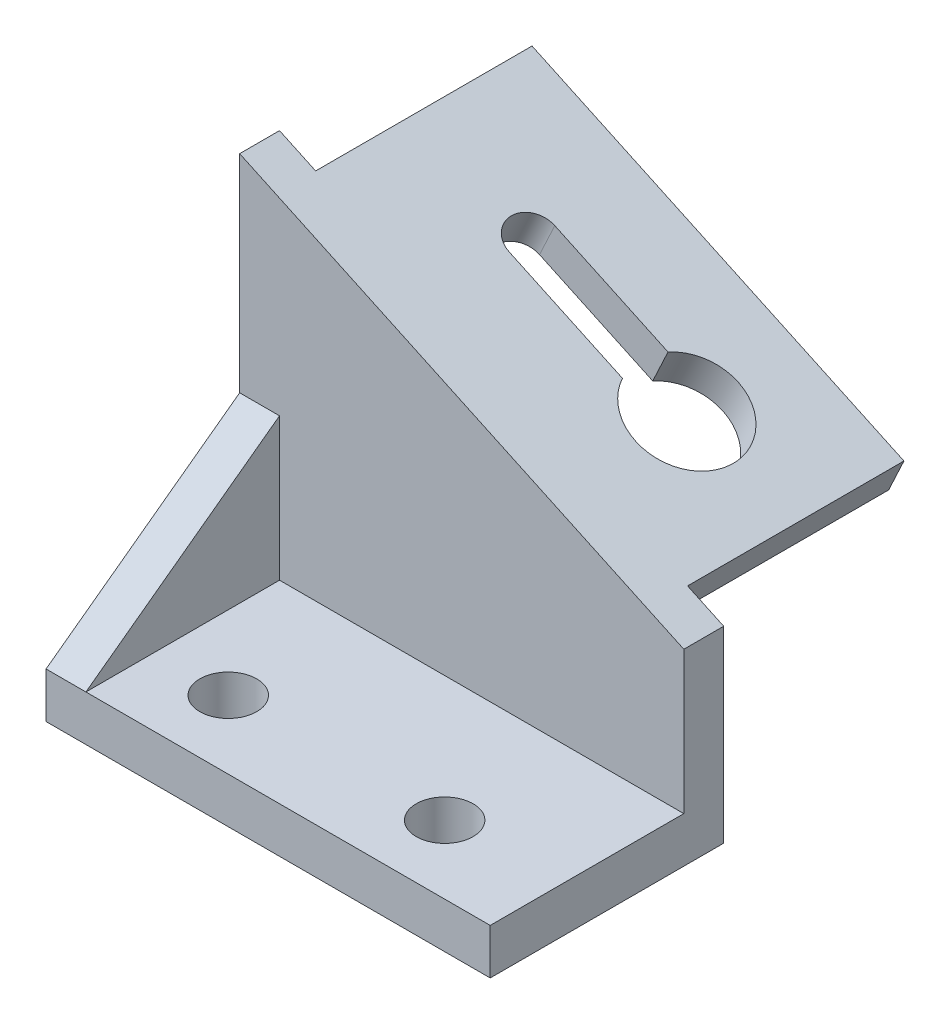
ISO-10303-21;
HEADER;
FILE_DESCRIPTION(('STEP AP214'),'2;1');
FILE_NAME('part.step','',(''),(''),'','','');
FILE_SCHEMA(('AUTOMOTIVE_DESIGN { 1 0 10303 214 1 1 1 1 }'));
ENDSEC;
DATA;
#1=APPLICATION_CONTEXT('core data for automotive mechanical design processes');
#2=APPLICATION_PROTOCOL_DEFINITION('international standard','automotive_design',2000,#1);
#3=PRODUCT_CONTEXT('',#1,'mechanical');
#4=PRODUCT('Part','Part','',(#3));
#5=PRODUCT_RELATED_PRODUCT_CATEGORY('part','',(#4));
#6=PRODUCT_DEFINITION_FORMATION('','',#4);
#7=PRODUCT_DEFINITION_CONTEXT('part definition',#1,'design');
#8=PRODUCT_DEFINITION('design','',#6,#7);
#9=PRODUCT_DEFINITION_SHAPE('','',#8);
#10=(LENGTH_UNIT() NAMED_UNIT(*) SI_UNIT(.MILLI.,.METRE.));
#11=(NAMED_UNIT(*) PLANE_ANGLE_UNIT() SI_UNIT($,.RADIAN.));
#12=(NAMED_UNIT(*) SI_UNIT($,.STERADIAN.) SOLID_ANGLE_UNIT());
#13=UNCERTAINTY_MEASURE_WITH_UNIT(LENGTH_MEASURE(1.E-05),#10,'distance_accuracy_value','');
#14=(GEOMETRIC_REPRESENTATION_CONTEXT(3) GLOBAL_UNCERTAINTY_ASSIGNED_CONTEXT((#13)) GLOBAL_UNIT_ASSIGNED_CONTEXT((#10,
#11,#12)) REPRESENTATION_CONTEXT('',''));
#15=CARTESIAN_POINT('',(0.,0.,0.));
#16=DIRECTION('',(0.,0.,1.));
#17=DIRECTION('',(1.,0.,0.));
#18=AXIS2_PLACEMENT_3D('',#15,#16,#17);
#19=CARTESIAN_POINT('',(-39.,8.,-16.5));
#20=DIRECTION('',(0.,0.,1.));
#21=DIRECTION('',(1.,0.,0.));
#22=AXIS2_PLACEMENT_3D('',#19,#20,#21);
#23=PLANE('',#22);
#24=DIRECTION('',(-0.90630778703665,0.4226182617407,0.));
#25=VECTOR('',#24,1.);
#26=CARTESIAN_POINT('',(39.,26.,-16.5));
#27=LINE('',#26,#25);
#28=CARTESIAN_POINT('',(29.974689939827,30.208571198282,-16.5));
#29=VERTEX_POINT('',#28);
#30=CARTESIAN_POINT('',(-35.3370010416599,60.6639128700022,-16.5));
#31=VERTEX_POINT('',#30);
#32=EDGE_CURVE('E205',#29,#31,#27,.T.);
#33=ORIENTED_EDGE('',*,*,#32,.F.);
#34=DIRECTION('',(0.4226182617407,0.906307787036649,0.));
#35=VECTOR('',#34,1.);
#36=CARTESIAN_POINT('',(16.5963515445968,1.51863192479222,-16.5));
#37=LINE('',#36,#35);
#38=CARTESIAN_POINT('',(32.6558454907434,35.9583278321849,-16.5));
#39=VERTEX_POINT('',#38);
#40=EDGE_CURVE('E195',#29,#39,#37,.T.);
#41=ORIENTED_EDGE('',*,*,#40,.T.);
#42=DIRECTION('',(0.90630778703665,-0.4226182617407,0.));
#43=VECTOR('',#42,1.);
#44=CARTESIAN_POINT('',(41.6811555509164,31.7497566339029,-16.5));
#45=LINE('',#44,#43);
#46=CARTESIAN_POINT('',(39.,33.,-16.5));
#47=VERTEX_POINT('',#46);
#48=EDGE_CURVE('E189',#39,#47,#45,.T.);
#49=ORIENTED_EDGE('',*,*,#48,.T.);
#50=DIRECTION('',(0.,-1.,0.));
#51=VECTOR('',#50,1.);
#52=CARTESIAN_POINT('',(39.,8.,-16.5));
#53=LINE('',#52,#51);
#54=CARTESIAN_POINT('',(39.,0.,-16.5));
#55=VERTEX_POINT('',#54);
#56=EDGE_CURVE('E276',#47,#55,#53,.T.);
#57=ORIENTED_EDGE('',*,*,#56,.T.);
#58=DIRECTION('',(-1.,0.,0.));
#59=VECTOR('',#58,1.);
#60=CARTESIAN_POINT('',(-39.,0.,-16.5));
#61=LINE('',#60,#59);
#62=CARTESIAN_POINT('',(-39.,0.,-16.5));
#63=VERTEX_POINT('',#62);
#64=EDGE_CURVE('E266',#55,#63,#61,.T.);
#65=ORIENTED_EDGE('',*,*,#64,.T.);
#66=DIRECTION('',(0.,-1.,0.));
#67=VECTOR('',#66,1.);
#68=CARTESIAN_POINT('',(-39.,8.,-16.5));
#69=LINE('',#68,#67);
#70=CARTESIAN_POINT('',(-39.,69.37199733609,-16.5));
#71=VERTEX_POINT('',#70);
#72=EDGE_CURVE('E277',#71,#63,#69,.T.);
#73=ORIENTED_EDGE('',*,*,#72,.F.);
#74=DIRECTION('',(0.90630778703665,-0.4226182617407,0.));
#75=VECTOR('',#74,1.);
#76=CARTESIAN_POINT('',(-32.6558454907434,66.4136695039051,-16.5));
#77=LINE('',#76,#75);
#78=CARTESIAN_POINT('',(-32.6558454907434,66.4136695039051,-16.5));
#79=VERTEX_POINT('',#78);
#80=EDGE_CURVE('E186',#71,#79,#77,.T.);
#81=ORIENTED_EDGE('',*,*,#80,.T.);
#82=DIRECTION('',(0.4226182617407,0.906307787036649,0.));
#83=VECTOR('',#82,1.);
#84=CARTESIAN_POINT('',(-48.7153394368901,31.9739735965124,-16.5));
#85=LINE('',#84,#83);
#86=EDGE_CURVE('E162',#31,#79,#85,.T.);
#87=ORIENTED_EDGE('',*,*,#86,.F.);
#88=EDGE_LOOP('',(#33,#41,#49,#57,#65,#73,#81,#87));
#89=FACE_BOUND('',#88,.T.);
#90=ADVANCED_FACE('F39',(#89),#23,.F.);
#91=CARTESIAN_POINT('',(0.,8.,0.));
#92=DIRECTION('',(0.,-1.,0.));
#93=DIRECTION('',(0.,0.,-1.));
#94=AXIS2_PLACEMENT_3D('',#91,#92,#93);
#95=PLANE('',#94);
#96=CARTESIAN_POINT('',(19.,8.,12.5));
#97=DIRECTION('',(0.,1.,0.));
#98=DIRECTION('',(0.,0.,1.));
#99=AXIS2_PLACEMENT_3D('',#96,#97,#98);
#100=CIRCLE('',#99,5.);
#101=CARTESIAN_POINT('',(19.,8.,17.5));
#102=VERTEX_POINT('',#101);
#103=EDGE_CURVE('E244',#102,#102,#100,.T.);
#104=ORIENTED_EDGE('',*,*,#103,.F.);
#105=EDGE_LOOP('',(#104));
#106=FACE_BOUND('',#105,.T.);
#107=CARTESIAN_POINT('',(-19.,8.,12.5));
#108=DIRECTION('',(0.,1.,0.));
#109=DIRECTION('',(0.,0.,1.));
#110=AXIS2_PLACEMENT_3D('',#107,#108,#109);
#111=CIRCLE('',#110,5.);
#112=CARTESIAN_POINT('',(-19.,8.,17.5));
#113=VERTEX_POINT('',#112);
#114=EDGE_CURVE('E252',#113,#113,#111,.T.);
#115=ORIENTED_EDGE('',*,*,#114,.F.);
#116=EDGE_LOOP('',(#115));
#117=FACE_BOUND('',#116,.T.);
#118=DIRECTION('',(1.,0.,0.));
#119=VECTOR('',#118,1.);
#120=CARTESIAN_POINT('',(-39.,8.,-9.50000000000001));
#121=LINE('',#120,#119);
#122=CARTESIAN_POINT('',(-32.,8.,-9.50000000000001));
#123=VERTEX_POINT('',#122);
#124=CARTESIAN_POINT('',(39.,8.,-9.50000000000001));
#125=VERTEX_POINT('',#124);
#126=EDGE_CURVE('E233',#123,#125,#121,.T.);
#127=ORIENTED_EDGE('',*,*,#126,.F.);
#128=DIRECTION('',(0.,0.,1.));
#129=VECTOR('',#128,1.);
#130=CARTESIAN_POINT('',(-32.,8.,-16.5));
#131=LINE('',#130,#129);
#132=CARTESIAN_POINT('',(-32.,8.,24.5));
#133=VERTEX_POINT('',#132);
#134=EDGE_CURVE('E241',#123,#133,#131,.T.);
#135=ORIENTED_EDGE('',*,*,#134,.T.);
#136=DIRECTION('',(1.,0.,0.));
#137=VECTOR('',#136,1.);
#138=CARTESIAN_POINT('',(-39.,8.,24.5));
#139=LINE('',#138,#137);
#140=CARTESIAN_POINT('',(39.,8.,24.5));
#141=VERTEX_POINT('',#140);
#142=EDGE_CURVE('E258',#133,#141,#139,.T.);
#143=ORIENTED_EDGE('',*,*,#142,.T.);
#144=DIRECTION('',(0.,0.,-1.));
#145=VECTOR('',#144,1.);
#146=CARTESIAN_POINT('',(39.,8.,24.5));
#147=LINE('',#146,#145);
#148=EDGE_CURVE('E260',#141,#125,#147,.T.);
#149=ORIENTED_EDGE('',*,*,#148,.T.);
#150=EDGE_LOOP('',(#127,#135,#143,#149));
#151=FACE_BOUND('',#150,.T.);
#152=ADVANCED_FACE('F325',(#106,#117,#151),#95,.F.);
#153=CARTESIAN_POINT('',(-32.,46.,-16.5));
#154=DIRECTION('',(1.,0.,0.));
#155=DIRECTION('',(0.,0.,-1.));
#156=AXIS2_PLACEMENT_3D('',#153,#154,#155);
#157=PLANE('',#156);
#158=DIRECTION('',(0.,0.592390450477518,-0.805651012649425));
#159=VECTOR('',#158,1.);
#160=CARTESIAN_POINT('',(-32.,33.,-9.50000000000001));
#161=LINE('',#160,#159);
#162=CARTESIAN_POINT('',(-32.,33.,-9.50000000000001));
#163=VERTEX_POINT('',#162);
#164=EDGE_CURVE('E218',#133,#163,#161,.T.);
#165=ORIENTED_EDGE('',*,*,#164,.F.);
#166=ORIENTED_EDGE('',*,*,#134,.F.);
#167=DIRECTION('',(0.,1.,0.));
#168=VECTOR('',#167,1.);
#169=CARTESIAN_POINT('',(-32.,46.,-9.50000000000001));
#170=LINE('',#169,#168);
#171=EDGE_CURVE('E238',#123,#163,#170,.T.);
#172=ORIENTED_EDGE('',*,*,#171,.T.);
#173=EDGE_LOOP('',(#165,#166,#172));
#174=FACE_BOUND('',#173,.T.);
#175=ADVANCED_FACE('F319',(#174),#157,.T.);
#176=CARTESIAN_POINT('',(0.,0.,0.));
#177=DIRECTION('',(0.,-1.,0.));
#178=DIRECTION('',(0.,0.,-1.));
#179=AXIS2_PLACEMENT_3D('',#176,#177,#178);
#180=PLANE('',#179);
#181=CARTESIAN_POINT('',(-19.,0.,12.5));
#182=DIRECTION('',(0.,1.,0.));
#183=DIRECTION('',(0.,0.,1.));
#184=AXIS2_PLACEMENT_3D('',#181,#182,#183);
#185=CIRCLE('',#184,5.);
#186=CARTESIAN_POINT('',(-19.,0.,17.5));
#187=VERTEX_POINT('',#186);
#188=EDGE_CURVE('E247',#187,#187,#185,.T.);
#189=ORIENTED_EDGE('',*,*,#188,.T.);
#190=EDGE_LOOP('',(#189));
#191=FACE_BOUND('',#190,.T.);
#192=DIRECTION('',(0.,0.,-1.));
#193=VECTOR('',#192,1.);
#194=CARTESIAN_POINT('',(39.,0.,24.5));
#195=LINE('',#194,#193);
#196=CARTESIAN_POINT('',(39.,0.,24.5));
#197=VERTEX_POINT('',#196);
#198=EDGE_CURVE('E251',#197,#55,#195,.T.);
#199=ORIENTED_EDGE('',*,*,#198,.F.);
#200=DIRECTION('',(1.,0.,0.));
#201=VECTOR('',#200,1.);
#202=CARTESIAN_POINT('',(-39.,0.,24.5));
#203=LINE('',#202,#201);
#204=CARTESIAN_POINT('',(-39.,0.,24.5));
#205=VERTEX_POINT('',#204);
#206=EDGE_CURVE('E262',#205,#197,#203,.T.);
#207=ORIENTED_EDGE('',*,*,#206,.F.);
#208=DIRECTION('',(0.,0.,1.));
#209=VECTOR('',#208,1.);
#210=CARTESIAN_POINT('',(-39.,0.,24.5));
#211=LINE('',#210,#209);
#212=EDGE_CURVE('E269',#63,#205,#211,.T.);
#213=ORIENTED_EDGE('',*,*,#212,.F.);
#214=ORIENTED_EDGE('',*,*,#64,.F.);
#215=EDGE_LOOP('',(#199,#207,#213,#214));
#216=FACE_BOUND('',#215,.T.);
#217=CARTESIAN_POINT('',(19.,0.,12.5));
#218=DIRECTION('',(0.,1.,0.));
#219=DIRECTION('',(0.,0.,1.));
#220=AXIS2_PLACEMENT_3D('',#217,#218,#219);
#221=CIRCLE('',#220,5.);
#222=CARTESIAN_POINT('',(19.,0.,17.5));
#223=VERTEX_POINT('',#222);
#224=EDGE_CURVE('E242',#223,#223,#221,.T.);
#225=ORIENTED_EDGE('',*,*,#224,.T.);
#226=EDGE_LOOP('',(#225));
#227=FACE_BOUND('',#226,.T.);
#228=ADVANCED_FACE('F331',(#191,#216,#227),#180,.T.);
#229=CARTESIAN_POINT('',(39.,8.,24.5));
#230=DIRECTION('',(-1.,0.,0.));
#231=DIRECTION('',(0.,0.,1.));
#232=AXIS2_PLACEMENT_3D('',#229,#230,#231);
#233=PLANE('',#232);
#234=ORIENTED_EDGE('',*,*,#56,.F.);
#235=DIRECTION('',(0.,0.,1.));
#236=VECTOR('',#235,1.);
#237=CARTESIAN_POINT('',(39.,33.,-67.5));
#238=LINE('',#237,#236);
#239=CARTESIAN_POINT('',(39.,33.,-9.50000000000001));
#240=VERTEX_POINT('',#239);
#241=EDGE_CURVE('E219',#47,#240,#238,.T.);
#242=ORIENTED_EDGE('',*,*,#241,.T.);
#243=DIRECTION('',(0.,-1.,0.));
#244=VECTOR('',#243,1.);
#245=CARTESIAN_POINT('',(39.,90.,-9.50000000000001));
#246=LINE('',#245,#244);
#247=EDGE_CURVE('E234',#240,#125,#246,.T.);
#248=ORIENTED_EDGE('',*,*,#247,.T.);
#249=ORIENTED_EDGE('',*,*,#148,.F.);
#250=DIRECTION('',(0.,-1.,0.));
#251=VECTOR('',#250,1.);
#252=CARTESIAN_POINT('',(39.,8.,24.5));
#253=LINE('',#252,#251);
#254=EDGE_CURVE('E264',#141,#197,#253,.T.);
#255=ORIENTED_EDGE('',*,*,#254,.T.);
#256=ORIENTED_EDGE('',*,*,#198,.T.);
#257=EDGE_LOOP('',(#234,#242,#248,#249,#255,#256));
#258=FACE_BOUND('',#257,.T.);
#259=ADVANCED_FACE('F41',(#258),#233,.F.);
#260=CARTESIAN_POINT('',(-39.,8.,24.5));
#261=DIRECTION('',(1.,0.,0.));
#262=DIRECTION('',(0.,0.,-1.));
#263=AXIS2_PLACEMENT_3D('',#260,#261,#262);
#264=PLANE('',#263);
#265=DIRECTION('',(0.,0.,1.));
#266=VECTOR('',#265,1.);
#267=CARTESIAN_POINT('',(-39.,69.37199733609,-67.5));
#268=LINE('',#267,#266);
#269=CARTESIAN_POINT('',(-39.,69.37199733609,-9.50000000000001));
#270=VERTEX_POINT('',#269);
#271=EDGE_CURVE('E220',#71,#270,#268,.T.);
#272=ORIENTED_EDGE('',*,*,#271,.F.);
#273=ORIENTED_EDGE('',*,*,#72,.T.);
#274=ORIENTED_EDGE('',*,*,#212,.T.);
#275=DIRECTION('',(0.,-1.,0.));
#276=VECTOR('',#275,1.);
#277=CARTESIAN_POINT('',(-39.,8.,24.5));
#278=LINE('',#277,#276);
#279=CARTESIAN_POINT('',(-39.,8.,24.5));
#280=VERTEX_POINT('',#279);
#281=EDGE_CURVE('E274',#280,#205,#278,.T.);
#282=ORIENTED_EDGE('',*,*,#281,.F.);
#283=DIRECTION('',(0.,0.592390450477518,-0.805651012649425));
#284=VECTOR('',#283,1.);
#285=CARTESIAN_POINT('',(-39.,8.00000000000001,24.5));
#286=LINE('',#285,#284);
#287=CARTESIAN_POINT('',(-39.,33.,-9.5));
#288=VERTEX_POINT('',#287);
#289=EDGE_CURVE('E227',#280,#288,#286,.T.);
#290=ORIENTED_EDGE('',*,*,#289,.T.);
#291=DIRECTION('',(0.,-1.,0.));
#292=VECTOR('',#291,1.);
#293=CARTESIAN_POINT('',(-39.,90.,-9.50000000000001));
#294=LINE('',#293,#292);
#295=EDGE_CURVE('E236',#270,#288,#294,.T.);
#296=ORIENTED_EDGE('',*,*,#295,.F.);
#297=EDGE_LOOP('',(#272,#273,#274,#282,#290,#296));
#298=FACE_BOUND('',#297,.T.);
#299=ADVANCED_FACE('F304',(#298),#264,.F.);
#300=CARTESIAN_POINT('',(-39.,8.,24.5));
#301=DIRECTION('',(0.,0.,-1.));
#302=DIRECTION('',(-1.,0.,0.));
#303=AXIS2_PLACEMENT_3D('',#300,#301,#302);
#304=PLANE('',#303);
#305=ORIENTED_EDGE('',*,*,#142,.F.);
#306=DIRECTION('',(1.,0.,0.));
#307=VECTOR('',#306,1.);
#308=CARTESIAN_POINT('',(-90.,8.,24.5));
#309=LINE('',#308,#307);
#310=EDGE_CURVE('E224',#280,#133,#309,.T.);
#311=ORIENTED_EDGE('',*,*,#310,.F.);
#312=ORIENTED_EDGE('',*,*,#281,.T.);
#313=ORIENTED_EDGE('',*,*,#206,.T.);
#314=ORIENTED_EDGE('',*,*,#254,.F.);
#315=EDGE_LOOP('',(#305,#311,#312,#313,#314));
#316=FACE_BOUND('',#315,.T.);
#317=ADVANCED_FACE('F323',(#316),#304,.F.);
#318=CARTESIAN_POINT('',(-19.,8.,12.5));
#319=DIRECTION('',(0.,-1.,0.));
#320=DIRECTION('',(0.,0.,-1.));
#321=AXIS2_PLACEMENT_3D('',#318,#319,#320);
#322=CYLINDRICAL_SURFACE('',#321,5.);
#323=ORIENTED_EDGE('',*,*,#114,.T.);
#324=EDGE_LOOP('',(#323));
#325=FACE_BOUND('',#324,.T.);
#326=ORIENTED_EDGE('',*,*,#188,.F.);
#327=EDGE_LOOP('',(#326));
#328=FACE_BOUND('',#327,.T.);
#329=ADVANCED_FACE('F338',(#325,#328),#322,.F.);
#330=CARTESIAN_POINT('',(19.,8.,12.5));
#331=DIRECTION('',(0.,-1.,0.));
#332=DIRECTION('',(0.,0.,-1.));
#333=AXIS2_PLACEMENT_3D('',#330,#331,#332);
#334=CYLINDRICAL_SURFACE('',#333,5.);
#335=ORIENTED_EDGE('',*,*,#103,.T.);
#336=EDGE_LOOP('',(#335));
#337=FACE_BOUND('',#336,.T.);
#338=ORIENTED_EDGE('',*,*,#224,.F.);
#339=EDGE_LOOP('',(#338));
#340=FACE_BOUND('',#339,.T.);
#341=ADVANCED_FACE('F336',(#337,#340),#334,.F.);
#342=CARTESIAN_POINT('',(-39.,90.,-9.50000000000001));
#343=DIRECTION('',(0.,0.,-1.));
#344=DIRECTION('',(-1.,0.,0.));
#345=AXIS2_PLACEMENT_3D('',#342,#343,#344);
#346=PLANE('',#345);
#347=ORIENTED_EDGE('',*,*,#247,.F.);
#348=DIRECTION('',(0.90630778703665,-0.4226182617407,0.));
#349=VECTOR('',#348,1.);
#350=CARTESIAN_POINT('',(-39.,69.37199733609,-9.50000000000001));
#351=LINE('',#350,#349);
#352=EDGE_CURVE('E215',#270,#240,#351,.T.);
#353=ORIENTED_EDGE('',*,*,#352,.F.);
#354=ORIENTED_EDGE('',*,*,#295,.T.);
#355=DIRECTION('',(1.,0.,0.));
#356=VECTOR('',#355,1.);
#357=CARTESIAN_POINT('',(-90.,33.,-9.49999999999999));
#358=LINE('',#357,#356);
#359=EDGE_CURVE('E223',#288,#163,#358,.T.);
#360=ORIENTED_EDGE('',*,*,#359,.T.);
#361=ORIENTED_EDGE('',*,*,#171,.F.);
#362=ORIENTED_EDGE('',*,*,#126,.T.);
#363=EDGE_LOOP('',(#347,#353,#354,#360,#361,#362));
#364=FACE_BOUND('',#363,.T.);
#365=ADVANCED_FACE('F311',(#364),#346,.F.);
#366=CARTESIAN_POINT('',(-90.,33.,-9.49999999999999));
#367=DIRECTION('',(0.,-0.805651012649425,-0.592390450477518));
#368=DIRECTION('',(0.,0.592390450477518,-0.805651012649425));
#369=AXIS2_PLACEMENT_3D('',#366,#367,#368);
#370=PLANE('',#369);
#371=ORIENTED_EDGE('',*,*,#310,.T.);
#372=ORIENTED_EDGE('',*,*,#164,.T.);
#373=ORIENTED_EDGE('',*,*,#359,.F.);
#374=ORIENTED_EDGE('',*,*,#289,.F.);
#375=EDGE_LOOP('',(#371,#372,#373,#374));
#376=FACE_BOUND('',#375,.T.);
#377=ADVANCED_FACE('F312',(#376),#370,.F.);
#378=CARTESIAN_POINT('',(-39.,69.37199733609,-67.5));
#379=DIRECTION('',(-0.4226182617407,-0.90630778703665,0.));
#380=DIRECTION('',(0.90630778703665,-0.4226182617407,0.));
#381=AXIS2_PLACEMENT_3D('',#378,#379,#380);
#382=PLANE('',#381);
#383=DIRECTION('',(0.906307787036649,-0.4226182617407,0.));
#384=VECTOR('',#383,1.);
#385=CARTESIAN_POINT('',(-12.659543861089,57.0892409192199,-30.5));
#386=LINE('',#385,#384);
#387=CARTESIAN_POINT('',(-12.6595438610891,57.0892409192199,-30.5));
#388=VERTEX_POINT('',#387);
#389=CARTESIAN_POINT('',(7.22280277163092,47.8179504222903,-30.5));
#390=VERTEX_POINT('',#389);
#391=EDGE_CURVE('E167',#388,#390,#386,.T.);
#392=ORIENTED_EDGE('',*,*,#391,.F.);
#393=CARTESIAN_POINT('',(-12.659543861089,57.0892409192199,-34.5));
#394=DIRECTION('',(0.4226182617407,0.906307787036649,0.));
#395=DIRECTION('',(-0.906307787036649,0.4226182617407,0.));
#396=AXIS2_PLACEMENT_3D('',#393,#394,#395);
#397=CIRCLE('',#396,4.00000000000001);
#398=CARTESIAN_POINT('',(-12.659543861089,57.0892409192199,-38.5));
#399=VERTEX_POINT('',#398);
#400=EDGE_CURVE('E53',#399,#388,#397,.T.);
#401=ORIENTED_EDGE('',*,*,#400,.F.);
#402=DIRECTION('',(-0.906307787036649,0.4226182617407,0.));
#403=VECTOR('',#402,1.);
#404=CARTESIAN_POINT('',(-12.659543861089,57.0892409192199,-38.5));
#405=LINE('',#404,#403);
#406=CARTESIAN_POINT('',(7.22280277163093,47.8179504222903,-38.5));
#407=VERTEX_POINT('',#406);
#408=EDGE_CURVE('E156',#407,#399,#405,.T.);
#409=ORIENTED_EDGE('',*,*,#408,.F.);
#410=CARTESIAN_POINT('',(14.5296897500105,44.4106930669989,-34.5));
#411=DIRECTION('',(0.4226182617407,0.906307787036649,0.));
#412=DIRECTION('',(-0.906307787036649,0.4226182617407,0.));
#413=AXIS2_PLACEMENT_3D('',#410,#411,#412);
#414=CIRCLE('',#413,9.);
#415=EDGE_CURVE('E176',#390,#407,#414,.T.);
#416=ORIENTED_EDGE('',*,*,#415,.F.);
#417=EDGE_LOOP('',(#392,#401,#409,#416));
#418=FACE_BOUND('',#417,.T.);
#419=ORIENTED_EDGE('',*,*,#241,.F.);
#420=ORIENTED_EDGE('',*,*,#48,.F.);
#421=DIRECTION('',(0.,0.,1.));
#422=VECTOR('',#421,1.);
#423=CARTESIAN_POINT('',(32.6558454907434,35.9583278321849,-16.5));
#424=LINE('',#423,#422);
#425=CARTESIAN_POINT('',(32.6558454907434,35.9583278321849,-54.5));
#426=VERTEX_POINT('',#425);
#427=EDGE_CURVE('E184',#426,#39,#424,.T.);
#428=ORIENTED_EDGE('',*,*,#427,.F.);
#429=DIRECTION('',(0.90630778703665,-0.4226182617407,0.));
#430=VECTOR('',#429,1.);
#431=CARTESIAN_POINT('',(39.,33.,-54.5));
#432=LINE('',#431,#430);
#433=CARTESIAN_POINT('',(-32.6558454907435,66.4136695039051,-54.5));
#434=VERTEX_POINT('',#433);
#435=EDGE_CURVE('E209',#434,#426,#432,.T.);
#436=ORIENTED_EDGE('',*,*,#435,.F.);
#437=DIRECTION('',(0.,0.,-1.));
#438=VECTOR('',#437,1.);
#439=CARTESIAN_POINT('',(-32.6558454907434,66.4136695039051,-54.5));
#440=LINE('',#439,#438);
#441=EDGE_CURVE('E197',#79,#434,#440,.T.);
#442=ORIENTED_EDGE('',*,*,#441,.F.);
#443=ORIENTED_EDGE('',*,*,#80,.F.);
#444=ORIENTED_EDGE('',*,*,#271,.T.);
#445=ORIENTED_EDGE('',*,*,#352,.T.);
#446=EDGE_LOOP('',(#419,#420,#428,#436,#442,#443,#444,#445));
#447=FACE_BOUND('',#446,.T.);
#448=ADVANCED_FACE('F300',(#418,#447),#382,.F.);
#449=CARTESIAN_POINT('',(39.,26.,-54.5));
#450=DIRECTION('',(0.4226182617407,0.906307787036649,0.));
#451=DIRECTION('',(-0.90630778703665,0.4226182617407,0.));
#452=AXIS2_PLACEMENT_3D('',#449,#450,#451);
#453=PLANE('',#452);
#454=DIRECTION('',(0.90630778703665,-0.4226182617407,0.));
#455=VECTOR('',#454,1.);
#456=CARTESIAN_POINT('',(-15.3406994120055,51.339484285317,-38.5));
#457=LINE('',#456,#455);
#458=CARTESIAN_POINT('',(-15.3406994120055,51.339484285317,-38.5));
#459=VERTEX_POINT('',#458);
#460=CARTESIAN_POINT('',(4.5416472207145,42.0681937883874,-38.5));
#461=VERTEX_POINT('',#460);
#462=EDGE_CURVE('E166',#459,#461,#457,.T.);
#463=ORIENTED_EDGE('',*,*,#462,.F.);
#464=CARTESIAN_POINT('',(-15.3406994120055,51.339484285317,-34.5));
#465=DIRECTION('',(0.4226182617407,0.906307787036649,0.));
#466=DIRECTION('',(-0.90630778703665,0.4226182617407,0.));
#467=AXIS2_PLACEMENT_3D('',#464,#465,#466);
#468=CIRCLE('',#467,4.00000000000001);
#469=CARTESIAN_POINT('',(-15.3406994120055,51.339484285317,-30.5));
#470=VERTEX_POINT('',#469);
#471=EDGE_CURVE('E148',#470,#459,#468,.F.);
#472=ORIENTED_EDGE('',*,*,#471,.F.);
#473=DIRECTION('',(-0.90630778703665,0.4226182617407,0.));
#474=VECTOR('',#473,1.);
#475=CARTESIAN_POINT('',(-15.3406994120055,51.339484285317,-30.5));
#476=LINE('',#475,#474);
#477=CARTESIAN_POINT('',(4.54164722071449,42.0681937883875,-30.5));
#478=VERTEX_POINT('',#477);
#479=EDGE_CURVE('E158',#478,#470,#476,.T.);
#480=ORIENTED_EDGE('',*,*,#479,.F.);
#481=CARTESIAN_POINT('',(11.848534199094,38.660936433096,-34.5));
#482=DIRECTION('',(0.4226182617407,0.906307787036649,0.));
#483=DIRECTION('',(-0.90630778703665,0.4226182617407,0.));
#484=AXIS2_PLACEMENT_3D('',#481,#482,#483);
#485=CIRCLE('',#484,9.);
#486=EDGE_CURVE('E65',#461,#478,#485,.F.);
#487=ORIENTED_EDGE('',*,*,#486,.F.);
#488=EDGE_LOOP('',(#463,#472,#480,#487));
#489=FACE_BOUND('',#488,.T.);
#490=DIRECTION('',(-0.90630778703665,0.4226182617407,0.));
#491=VECTOR('',#490,1.);
#492=CARTESIAN_POINT('',(39.,26.,-54.5));
#493=LINE('',#492,#491);
#494=CARTESIAN_POINT('',(29.974689939827,30.208571198282,-54.5));
#495=VERTEX_POINT('',#494);
#496=CARTESIAN_POINT('',(-35.3370010416599,60.6639128700022,-54.5));
#497=VERTEX_POINT('',#496);
#498=EDGE_CURVE('E207',#495,#497,#493,.T.);
#499=ORIENTED_EDGE('',*,*,#498,.F.);
#500=DIRECTION('',(0.,0.,1.));
#501=VECTOR('',#500,1.);
#502=CARTESIAN_POINT('',(29.974689939827,30.208571198282,-54.5));
#503=LINE('',#502,#501);
#504=EDGE_CURVE('E202',#495,#29,#503,.T.);
#505=ORIENTED_EDGE('',*,*,#504,.T.);
#506=ORIENTED_EDGE('',*,*,#32,.T.);
#507=DIRECTION('',(0.,0.,-1.));
#508=VECTOR('',#507,1.);
#509=CARTESIAN_POINT('',(-35.3370010416599,60.6639128700022,-54.5));
#510=LINE('',#509,#508);
#511=EDGE_CURVE('E191',#31,#497,#510,.T.);
#512=ORIENTED_EDGE('',*,*,#511,.T.);
#513=EDGE_LOOP('',(#499,#505,#506,#512));
#514=FACE_BOUND('',#513,.T.);
#515=ADVANCED_FACE('F164',(#489,#514),#453,.F.);
#516=CARTESIAN_POINT('',(0.,0.,-54.5));
#517=DIRECTION('',(0.,0.,-1.));
#518=DIRECTION('',(-1.,0.,0.));
#519=AXIS2_PLACEMENT_3D('',#516,#517,#518);
#520=PLANE('',#519);
#521=DIRECTION('',(0.4226182617407,0.90630778703665,0.));
#522=VECTOR('',#521,1.);
#523=CARTESIAN_POINT('',(13.0504705681678,-6.08553436846307,-54.5));
#524=LINE('',#523,#522);
#525=EDGE_CURVE('E11',#495,#426,#524,.T.);
#526=ORIENTED_EDGE('',*,*,#525,.F.);
#527=ORIENTED_EDGE('',*,*,#498,.T.);
#528=DIRECTION('',(-0.4226182617407,-0.90630778703665,0.));
#529=VECTOR('',#528,1.);
#530=CARTESIAN_POINT('',(-52.2612204133191,24.3698073032571,-54.5));
#531=LINE('',#530,#529);
#532=EDGE_CURVE('E50',#434,#497,#531,.T.);
#533=ORIENTED_EDGE('',*,*,#532,.F.);
#534=ORIENTED_EDGE('',*,*,#435,.T.);
#535=EDGE_LOOP('',(#526,#527,#533,#534));
#536=FACE_BOUND('',#535,.T.);
#537=ADVANCED_FACE('F290',(#536),#520,.T.);
#538=CARTESIAN_POINT('',(-48.7153394368901,31.9739735965124,-54.5));
#539=DIRECTION('',(0.906307787036649,-0.4226182617407,0.));
#540=DIRECTION('',(0.4226182617407,0.90630778703665,0.));
#541=AXIS2_PLACEMENT_3D('',#538,#539,#540);
#542=PLANE('',#541);
#543=ORIENTED_EDGE('',*,*,#86,.T.);
#544=ORIENTED_EDGE('',*,*,#441,.T.);
#545=ORIENTED_EDGE('',*,*,#532,.T.);
#546=ORIENTED_EDGE('',*,*,#511,.F.);
#547=EDGE_LOOP('',(#543,#544,#545,#546));
#548=FACE_BOUND('',#547,.T.);
#549=ADVANCED_FACE('F285',(#548),#542,.F.);
#550=CARTESIAN_POINT('',(16.5963515445968,1.51863192479222,-16.5));
#551=DIRECTION('',(-0.906307787036649,0.4226182617407,0.));
#552=DIRECTION('',(-0.4226182617407,-0.90630778703665,0.));
#553=AXIS2_PLACEMENT_3D('',#550,#551,#552);
#554=PLANE('',#553);
#555=ORIENTED_EDGE('',*,*,#525,.T.);
#556=ORIENTED_EDGE('',*,*,#427,.T.);
#557=ORIENTED_EDGE('',*,*,#40,.F.);
#558=ORIENTED_EDGE('',*,*,#504,.F.);
#559=EDGE_LOOP('',(#555,#556,#557,#558));
#560=FACE_BOUND('',#559,.T.);
#561=ADVANCED_FACE('F291',(#560),#554,.F.);
#562=CARTESIAN_POINT('',(-39.2311220231939,0.106307661725459,-34.5));
#563=DIRECTION('',(0.4226182617407,0.906307787036649,0.));
#564=DIRECTION('',(-0.906307787036649,0.4226182617407,0.));
#565=AXIS2_PLACEMENT_3D('',#562,#563,#564);
#566=CYLINDRICAL_SURFACE('',#565,4.00000000000001);
#567=ORIENTED_EDGE('',*,*,#471,.T.);
#568=DIRECTION('',(0.4226182617407,0.906307787036649,0.));
#569=VECTOR('',#568,1.);
#570=CARTESIAN_POINT('',(-39.2311220231939,0.106307661725459,-38.5));
#571=LINE('',#570,#569);
#572=EDGE_CURVE('E161',#459,#399,#571,.T.);
#573=ORIENTED_EDGE('',*,*,#572,.T.);
#574=ORIENTED_EDGE('',*,*,#400,.T.);
#575=DIRECTION('',(0.4226182617407,0.906307787036649,0.));
#576=VECTOR('',#575,1.);
#577=CARTESIAN_POINT('',(-39.2311220231939,0.106307661725459,-30.5));
#578=LINE('',#577,#576);
#579=EDGE_CURVE('E147',#470,#388,#578,.T.);
#580=ORIENTED_EDGE('',*,*,#579,.F.);
#581=EDGE_LOOP('',(#567,#573,#574,#580));
#582=FACE_BOUND('',#581,.T.);
#583=ADVANCED_FACE('F149',(#582),#566,.F.);
#584=CARTESIAN_POINT('',(-39.2311220231939,0.106307661725459,-38.5));
#585=DIRECTION('',(0.,0.,-1.));
#586=DIRECTION('',(-1.,0.,0.));
#587=AXIS2_PLACEMENT_3D('',#584,#585,#586);
#588=PLANE('',#587);
#589=ORIENTED_EDGE('',*,*,#462,.T.);
#590=DIRECTION('',(0.4226182617407,0.906307787036649,0.));
#591=VECTOR('',#590,1.);
#592=CARTESIAN_POINT('',(-19.348775390474,-9.16498283520413,-38.5));
#593=LINE('',#592,#591);
#594=EDGE_CURVE('E185',#461,#407,#593,.T.);
#595=ORIENTED_EDGE('',*,*,#594,.T.);
#596=ORIENTED_EDGE('',*,*,#408,.T.);
#597=ORIENTED_EDGE('',*,*,#572,.F.);
#598=EDGE_LOOP('',(#589,#595,#596,#597));
#599=FACE_BOUND('',#598,.T.);
#600=ADVANCED_FACE('F484',(#599),#588,.F.);
#601=CARTESIAN_POINT('',(-12.0418884120944,-12.5722401904956,-34.5));
#602=DIRECTION('',(0.4226182617407,0.906307787036649,0.));
#603=DIRECTION('',(-0.906307787036649,0.4226182617407,0.));
#604=AXIS2_PLACEMENT_3D('',#601,#602,#603);
#605=CYLINDRICAL_SURFACE('',#604,9.);
#606=ORIENTED_EDGE('',*,*,#486,.T.);
#607=DIRECTION('',(0.4226182617407,0.906307787036649,0.));
#608=VECTOR('',#607,1.);
#609=CARTESIAN_POINT('',(-19.348775390474,-9.16498283520413,-30.5));
#610=LINE('',#609,#608);
#611=EDGE_CURVE('E153',#478,#390,#610,.T.);
#612=ORIENTED_EDGE('',*,*,#611,.T.);
#613=ORIENTED_EDGE('',*,*,#415,.T.);
#614=ORIENTED_EDGE('',*,*,#594,.F.);
#615=EDGE_LOOP('',(#606,#612,#613,#614));
#616=FACE_BOUND('',#615,.T.);
#617=ADVANCED_FACE('F493',(#616),#605,.F.);
#618=CARTESIAN_POINT('',(-39.2311220231939,0.106307661725459,-30.5));
#619=DIRECTION('',(0.,0.,1.));
#620=DIRECTION('',(1.,0.,0.));
#621=AXIS2_PLACEMENT_3D('',#618,#619,#620);
#622=PLANE('',#621);
#623=ORIENTED_EDGE('',*,*,#479,.T.);
#624=ORIENTED_EDGE('',*,*,#579,.T.);
#625=ORIENTED_EDGE('',*,*,#391,.T.);
#626=ORIENTED_EDGE('',*,*,#611,.F.);
#627=EDGE_LOOP('',(#623,#624,#625,#626));
#628=FACE_BOUND('',#627,.T.);
#629=ADVANCED_FACE('F160',(#628),#622,.F.);
#630=CLOSED_SHELL('',(#90,#152,#175,#228,#259,#299,#317,#329,#341,#365,#377,#448,#515,#537,#549,
#561,#583,#600,#617,#629));
#631=MANIFOLD_SOLID_BREP('B2',#630);
#632=ADVANCED_BREP_SHAPE_REPRESENTATION('',(#18,#631),#14);
#633=SHAPE_DEFINITION_REPRESENTATION(#9,#632);
ENDSEC;
END-ISO-10303-21;
